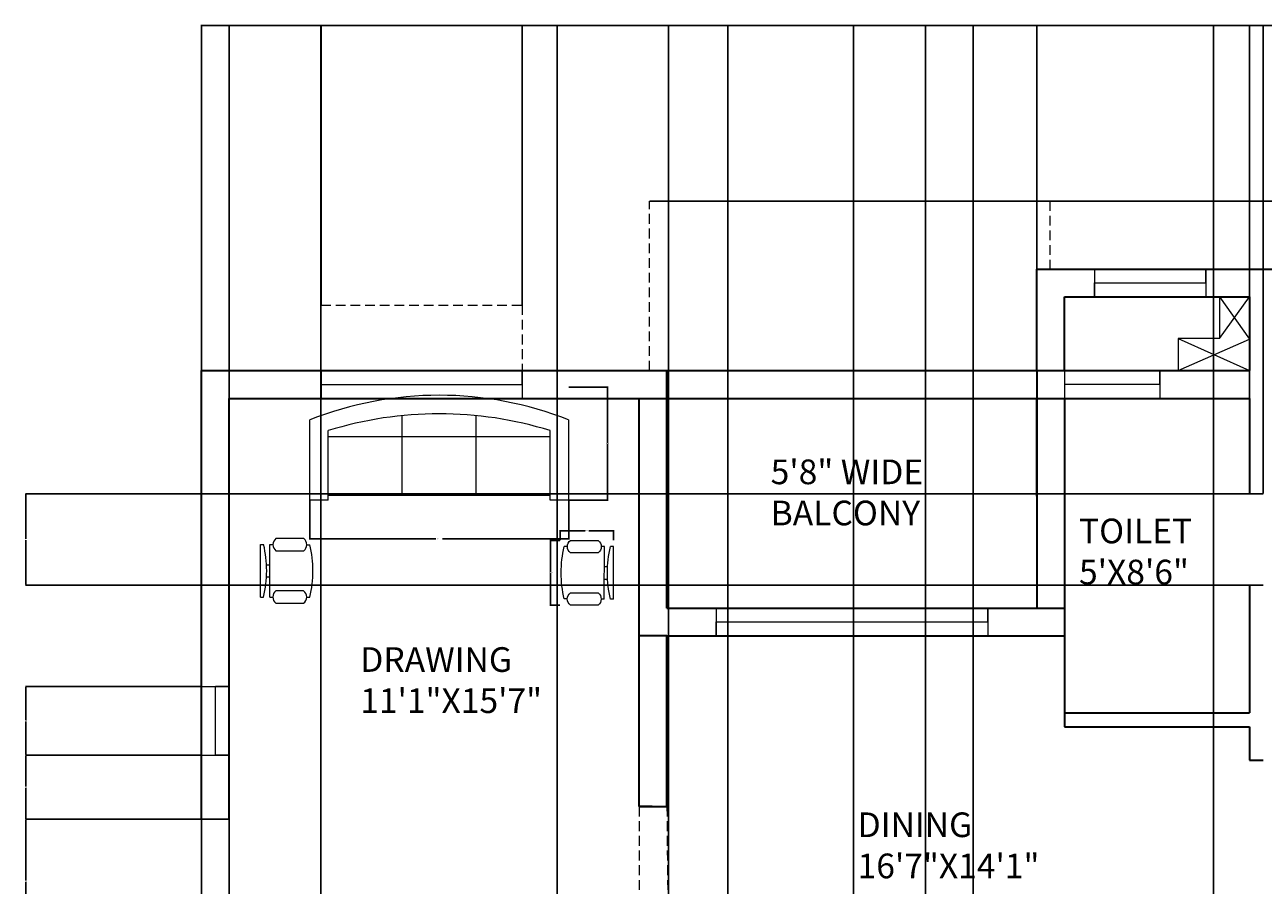
# Model space of a CAD drawing. Units: inches. Extents: x 276 to 912, y -567 to 621.
# Tile 6 of 7: x 276 to 678, y 342 to 621. Entities that reach past the tile are written whole.
import ezdxf

# ---------------------------------------------------------------- set-up
doc = ezdxf.new("R2010")
doc.units = ezdxf.units.IN
doc.linetypes.add('HIDDEN2', pattern=[4.7625, 3.175, -1.5875])
for name, color, linetype, lineweight in [('A-ANNO-DIMS', 2, 'Continuous', 18), ('A-AREA-IDEN', 7, 'Continuous', 18), ('A-DOOR', 3, 'Continuous', 25), ('A-FLOR-OVHD', 8, 'HIDDEN2', 13), ('A-FLOR-SHFT', 8, 'Continuous', 18), ('A-FURN', 8, 'Continuous', 18), ('A-GLAZ', 4, 'Continuous', 18), ('A-WALL', 7, 'Continuous', 35), ('A-WALL-HIDN', 8, 'HIDDEN2', 18)]:
    doc.layers.add(name, color=color, linetype=linetype, lineweight=lineweight)
doc.dimstyles.get("Standard").update_dxf_attribs({"dimtxt": 0.18, "dimasz": 0.18, "dimexe": 0.18, "dimexo": 0.0625, "dimgap": 0.09, "dimtad": 0, "dimtih": 1, "dimtoh": 1, "dimdec": 4, "dimzin": 0, "dimdsep": 46, "dimtxsty": 'Standard', "dimcen": 0.09, "dimadec": 0, "dimazin": 0, "dimtfac": 1, "dimtdec": 4, "dimtofl": 0, "dimtmove": 0, "dimatfit": 3, "dimfxl": 1, "dimtolj": 1, "dimtzin": 0, "dimarcsym": 0})

# ---------------------------------------------------------------- blocks, each defined once
blk = doc.blocks.new('Chair - Desk')
for p, q in [((-8.5, 0), (-8.5, -1)), ((-8.5, 0), (8.5, 0)), ((8.5, 0), (8.5, -1)), ((-8.5, -3), (-8.5, -4)), ((-8.5, -3), (8.5, -3)), ((-2, -3), (-2, -1.9355)), ((2, -1.9576), (2, -3)), ((8.5, -3), (8.5, -4)), ((-10.5, -5), (-10.5, -14)), ((-6.5, -14), (-6.5, -5)), ((6.5, -5), (6.5, -14)), ((10.5, -14), (10.5, -5)), ((-8.5, -15), (-8.5, -16)), ((8.5, -15), (8.5, -16))]:
    blk.add_line(p, q)
for centre, radius, start, end in [((-8.5, -6.5), 2.5, 36.8699, 143.1301), ((0, 34.625), 36.625, 256.5803, 283.4197), ((8.5, -6.5), 2.5, 36.8699, 143.1301), ((-8.5, -12.5), 2.5, 216.8699, 323.1301), ((0, 19.625), 36.625, 256.5803, 283.4197), ((8.5, -12.5), 2.5, 216.8699, 323.1301)]:
    blk.add_arc(centre, radius, start, end)
blk = doc.blocks.new('Sofa - Roundback 7 ft.')
for p, q in [((-12.00002, -32.4421), (-12.00003, -6.5971)), ((11.99997, -32.4421), (11.99998, -6.5971)), ((-36.000027, -34), (-36.000027, -11.4696)), ((35.99998, -34), (35.99998, -11.4696)), ((-35.999844, -13.3819), (35.9998, -13.3819)), ((-36.000027, -32.4421), (35.99998, -32.4421))]:
    blk.add_line(p, q)
for points in [[(-36.000027, -34), (-42.000027, -34), (-42.000027, -8)], [(41.99998, -8), (41.99998, -34), (35.99998, -34)]]:
    blk.add_lwpolyline(points)
for centre, radius, start, end in [((0, -114.25), 114.25, 68.43141, 111.5686), ((-0.00001, -127.1968), 121.1968, 72.72033, 107.2797)]:
    blk.add_arc(centre, radius, start, end)
blk = doc.blocks.new('DOOR-JAMB-4.5IN')
for p, q in [((0, 2.25), (0, 4.5)), ((0, 4.5), (0, 0))]:
    blk.add_line(p, q)
blk = doc.blocks.new('DOOR-JAMB-9IN')
for p, q in [((4.5, 0), (0, 0)), ((0, 0), (9, 0))]:
    blk.add_line(p, q)
blk = doc.blocks.new('*D14')
at = {"layer": 'A-ANNO-DIMS', "color": 0, "lineweight": -2, "transparency": 16777216}
for p, q in [((449.38, 454.26), (446.12, 454.27)), ((446.3, 454.09), (446.28, 443.95)), ((446.27, 433.45), (446.28, 443.59)), ((449.35, 433.26), (446.09, 433.27))]:
    blk.add_line(p, q, dxfattribs=at)
at = {"layer": 'A-ANNO-DIMS', "color": 0, "transparency": 16777216}
for points in [[(446.27, 454.09), (446.33, 454.09), (446.3, 454.27)], [(446.24, 433.45), (446.3, 433.45), (446.27, 433.27)]]:
    blk.add_solid(points, dxfattribs=at)
at = {"layer": 'Defpoints', "color": 0, "transparency": 16777216}
for p in [(446.3, 454.27), (449.45, 454.26), (449.42, 433.26)]:
    blk.add_point(p, dxfattribs=at)
at = {"layer": 'A-ANNO-DIMS', "color": 0, "transparency": 16777216, "insert": (446.28, 443.77), "char_height": 0.18, "attachment_point": 5}
blk.add_mtext('\\A1;CHAIR 21 TYP.', dxfattribs=at)
blk = doc.blocks.new('*D15')
at = {"layer": 'A-ANNO-DIMS', "color": 0, "lineweight": -2, "transparency": 16777216}
for p, q in [((449.45, 454.33), (449.45, 457.59)), ((449.63, 457.41), (457.52, 457.4)), ((466.6, 457.39), (458.72, 457.4)), ((466.78, 454.3), (466.78, 457.57))]:
    blk.add_line(p, q, dxfattribs=at)
at = {"layer": 'A-ANNO-DIMS', "color": 0, "transparency": 16777216}
for points in [[(449.63, 457.44), (449.63, 457.38), (449.45, 457.41)], [(466.6, 457.42), (466.6, 457.36), (466.78, 457.39)]]:
    blk.add_solid(points, dxfattribs=at)
at = {"layer": 'Defpoints', "color": 0, "transparency": 16777216}
for p in [(449.45, 454.26), (466.78, 457.39), (466.78, 454.24)]:
    blk.add_point(p, dxfattribs=at)
at = {"layer": 'A-ANNO-DIMS', "color": 0, "transparency": 16777216, "insert": (458.12, 457.4), "char_height": 0.18, "attachment_point": 5}
blk.add_mtext('\\A1;17 TYP.', dxfattribs=at)
blk = doc.blocks.new('*D20')
at = {"layer": 'A-ANNO-DIMS', "color": 0, "lineweight": -2, "transparency": 16777216}
for p, q in [((368.2, 467.26), (368.2, 454.55)), ((452.2, 467.26), (452.2, 454.55)), ((368.38, 454.73), (409.12, 454.73)), ((452.02, 454.73), (411.28, 454.73))]:
    blk.add_line(p, q, dxfattribs=at)
at = {"layer": 'A-ANNO-DIMS', "color": 0, "transparency": 16777216}
for points in [[(368.38, 454.76), (368.38, 454.7), (368.2, 454.73)], [(452.02, 454.76), (452.02, 454.7), (452.2, 454.73)]]:
    blk.add_solid(points, dxfattribs=at)
at = {"layer": 'Defpoints', "color": 0, "transparency": 16777216}
for p in [(368.2, 467.33), (452.2, 467.33), (452.2, 454.73)]:
    blk.add_point(p, dxfattribs=at)
at = {"layer": 'A-ANNO-DIMS', "color": 0, "transparency": 16777216, "insert": (410.2, 454.73), "char_height": 0.18, "attachment_point": 5}
blk.add_mtext('\\A1;SOFA 84 TYP.', dxfattribs=at)
blk = doc.blocks.new('*D21')
at = {"layer": 'A-ANNO-DIMS', "color": 0, "lineweight": -2, "transparency": 16777216}
for p, q in [((452.26, 503.99), (464.98, 503.99)), ((464.8, 503.81), (464.8, 485.84)), ((464.8, 467.51), (464.8, 485.48)), ((452.26, 467.33), (464.98, 467.33))]:
    blk.add_line(p, q, dxfattribs=at)
at = {"layer": 'A-ANNO-DIMS', "color": 0, "transparency": 16777216}
for points in [[(464.77, 503.81), (464.83, 503.81), (464.8, 503.99)], [(464.77, 467.51), (464.83, 467.51), (464.8, 467.33)]]:
    blk.add_solid(points, dxfattribs=at)
at = {"layer": 'Defpoints', "color": 0, "transparency": 16777216}
for p in [(452.2, 503.99), (464.8, 503.99), (452.2, 467.33)]:
    blk.add_point(p, dxfattribs=at)
at = {"layer": 'A-ANNO-DIMS', "color": 0, "transparency": 16777216, "insert": (464.8, 485.66), "char_height": 0.18, "attachment_point": 5}
blk.add_mtext('\\A1;37 TYP.', dxfattribs=at)
blk = doc.blocks.new('*D25')
at = {"layer": 'A-ANNO-DIMS', "color": 0, "lineweight": -2, "transparency": 16777216}
for p, q in [((478.5, 564.29), (911.39, 564.29)), ((911.21, 564.11), (911.21, 34.31)), ((911.21, -495.86), (911.21, 33.95)), ((582.98, -496.04), (911.39, -496.04))]:
    blk.add_line(p, q, dxfattribs=at)
at = {"layer": 'A-ANNO-DIMS', "color": 0, "transparency": 16777216}
for points in [[(911.18, 564.11), (911.24, 564.11), (911.21, 564.29)], [(911.18, -495.86), (911.24, -495.86), (911.21, -496.04)]]:
    blk.add_solid(points, dxfattribs=at)
at = {"layer": 'Defpoints', "color": 0, "transparency": 16777216}
for p in [(478.44, 564.29), (582.92, -496.04), (911.21, -496.04)]:
    blk.add_point(p, dxfattribs=at)
at = {"layer": 'A-ANNO-DIMS', "color": 0, "transparency": 16777216, "insert": (911.21, 34.13), "char_height": 0.18, "attachment_point": 5}
blk.add_mtext('\\A1;1060.3', dxfattribs=at)
blk = doc.blocks.new('*D27')
at = {"layer": 'A-ANNO-DIMS', "color": 0, "lineweight": -2, "transparency": 16777216}
for p, q in [((333.082179, 509.380751), (333.082179, 621.473746)), ((333.262179, 621.293746), (468.282179, 621.293746)), ((603.902179, 621.293746), (468.882179, 621.293746)), ((604.082179, 542.322551), (604.082179, 621.473746))]:
    blk.add_line(p, q, dxfattribs=at)
at = {"layer": 'A-ANNO-DIMS', "color": 0, "transparency": 16777216}
for points in [[(333.262179, 621.323746), (333.262179, 621.263746), (333.082179, 621.293746)], [(603.902179, 621.323746), (603.902179, 621.263746), (604.082179, 621.293746)]]:
    blk.add_solid(points, dxfattribs=at)
at = {"layer": 'Defpoints', "color": 0, "transparency": 16777216}
for p in [(604.082179, 621.293746), (604.082179, 542.260051), (333.082179, 509.318251)]:
    blk.add_point(p, dxfattribs=at)
at = {"layer": 'A-ANNO-DIMS', "color": 0, "transparency": 16777216, "insert": (468.582179, 621.293746), "char_height": 0.18, "attachment_point": 5}
blk.add_mtext('\\A1;271', dxfattribs=at)
blk = doc.blocks.new('*D28')
at = {"layer": 'A-ANNO-DIMS', "color": 0, "lineweight": -2, "transparency": 16777216}
for p, q in [((604.082179, 542.322551), (604.082179, 621.473746)), ((604.262179, 621.293746), (642.842179, 621.293746)), ((681.902179, 621.293746), (643.322179, 621.293746)), ((682.082179, 542.322551), (682.082179, 621.473746))]:
    blk.add_line(p, q, dxfattribs=at)
at = {"layer": 'A-ANNO-DIMS', "color": 0, "transparency": 16777216}
for points in [[(604.262179, 621.323746), (604.262179, 621.263746), (604.082179, 621.293746)], [(681.902179, 621.323746), (681.902179, 621.263746), (682.082179, 621.293746)]]:
    blk.add_solid(points, dxfattribs=at)
at = {"layer": 'Defpoints', "color": 0, "transparency": 16777216}
for p in [(682.082179, 621.293746), (604.082179, 542.260051), (682.082179, 542.260051)]:
    blk.add_point(p, dxfattribs=at)
at = {"layer": 'A-ANNO-DIMS', "color": 0, "transparency": 16777216, "insert": (643.082179, 621.293746), "char_height": 0.18, "attachment_point": 5}
blk.add_mtext('\\A1;78', dxfattribs=at)
blk = doc.blocks.new('*D37')
at = {"layer": 'A-ANNO-DIMS', "color": 0, "lineweight": -2, "transparency": 16777216}
for p, q in [((333.019679, 363.831643), (275.902179, 363.831643)), ((276.082179, 363.651643), (276.082179, 343.929428)), ((276.082179, 323.847213), (276.082179, 343.569428)), ((333.019679, 323.667213), (275.902179, 323.667213))]:
    blk.add_line(p, q, dxfattribs=at)
at = {"layer": 'A-ANNO-DIMS', "color": 0, "transparency": 16777216}
for points in [[(276.052179, 363.651643), (276.112179, 363.651643), (276.082179, 363.831643)], [(276.052179, 323.847213), (276.112179, 323.847213), (276.082179, 323.667213)]]:
    blk.add_solid(points, dxfattribs=at)
at = {"layer": 'Defpoints', "color": 0, "transparency": 16777216}
for p in [(276.082179, 363.831643), (333.082179, 363.831643), (333.082179, 323.667213)]:
    blk.add_point(p, dxfattribs=at)
at = {"layer": 'A-ANNO-DIMS', "color": 0, "transparency": 16777216, "insert": (276.082179, 343.749428), "char_height": 0.18, "attachment_point": 5}
blk.add_mtext('\\A1;40.164', dxfattribs=at)
blk = doc.blocks.new('*D39')
at = {"layer": 'A-ANNO-DIMS', "color": 0, "lineweight": -2, "transparency": 16777216}
for p, q in [((673.019679, 469.398472), (275.902179, 469.398472)), ((276.082179, 469.218472), (276.082179, 454.742779)), ((276.082179, 439.907086), (276.082179, 454.382779)), ((673.019679, 439.727086), (275.902179, 439.727086))]:
    blk.add_line(p, q, dxfattribs=at)
at = {"layer": 'A-ANNO-DIMS', "color": 0, "transparency": 16777216}
for points in [[(276.052179, 469.218472), (276.112179, 469.218472), (276.082179, 469.398472)], [(276.052179, 439.907086), (276.112179, 439.907086), (276.082179, 439.727086)]]:
    blk.add_solid(points, dxfattribs=at)
at = {"layer": 'Defpoints', "color": 0, "transparency": 16777216}
for p in [(276.082179, 469.398472), (673.082179, 469.398472), (673.082179, 439.727086)]:
    blk.add_point(p, dxfattribs=at)
at = {"layer": 'A-ANNO-DIMS', "color": 0, "transparency": 16777216, "insert": (276.082179, 454.562779), "char_height": 0.18, "attachment_point": 5}
blk.add_mtext('\\A1;29.67', dxfattribs=at)
blk = doc.blocks.new('*D40')
at = {"layer": 'A-ANNO-DIMS', "color": 0, "lineweight": -2, "transparency": 16777216}
for p, q in [((673.082179, 469.460972), (673.082179, 621.473746)), ((673.262179, 621.293746), (675.062179, 621.293746)), ((677.402179, 621.293746), (675.602179, 621.293746)), ((677.582179, 469.460972), (677.582179, 621.473746))]:
    blk.add_line(p, q, dxfattribs=at)
at = {"layer": 'A-ANNO-DIMS', "color": 0, "transparency": 16777216}
for points in [[(673.262179, 621.323746), (673.262179, 621.263746), (673.082179, 621.293746)], [(677.402179, 621.323746), (677.402179, 621.263746), (677.582179, 621.293746)]]:
    blk.add_solid(points, dxfattribs=at)
at = {"layer": 'Defpoints', "color": 0, "transparency": 16777216}
for p in [(677.582179, 621.293746), (673.082179, 469.398472), (677.582179, 469.398472)]:
    blk.add_point(p, dxfattribs=at)
at = {"layer": 'A-ANNO-DIMS', "color": 0, "transparency": 16777216, "insert": (675.332179, 621.293746), "char_height": 0.18, "attachment_point": 5}
blk.add_mtext('\\A1;4.5', dxfattribs=at)
blk = doc.blocks.new('*D41')
at = {"layer": 'A-ANNO-DIMS', "color": 0, "lineweight": -2, "transparency": 16777216}
for p, q in [((333.082179, 363.769143), (333.082179, -553.223061)), ((342.082179, 363.769143), (342.082179, -553.223061)), ((333.262179, -553.043061), (337.432179, -553.043061)), ((341.902179, -553.043061), (337.732179, -553.043061))]:
    blk.add_line(p, q, dxfattribs=at)
at = {"layer": 'A-ANNO-DIMS', "color": 0, "transparency": 16777216}
for points in [[(333.262179, -553.013061), (333.262179, -553.073061), (333.082179, -553.043061)], [(341.902179, -553.013061), (341.902179, -553.073061), (342.082179, -553.043061)]]:
    blk.add_solid(points, dxfattribs=at)
at = {"layer": 'Defpoints', "color": 0, "transparency": 16777216}
for p in [(333.082179, 363.831643), (342.082179, 363.831643), (342.082179, -553.043061)]:
    blk.add_point(p, dxfattribs=at)
at = {"layer": 'A-ANNO-DIMS', "color": 0, "transparency": 16777216, "insert": (337.582179, -553.043061), "char_height": 0.18, "attachment_point": 5}
blk.add_mtext('\\A1;9', dxfattribs=at)
blk = doc.blocks.new('*D42')
at = {"layer": 'A-ANNO-DIMS', "color": 0, "lineweight": -2, "transparency": 16777216}
for p, q in [((484.582179, 267.783946), (484.582179, 621.473746)), ((484.762179, 621.293746), (514.357179, 621.293746)), ((544.402179, 621.293746), (514.807179, 621.293746)), ((544.582179, 267.783946), (544.582179, 621.473746))]:
    blk.add_line(p, q, dxfattribs=at)
at = {"layer": 'A-ANNO-DIMS', "color": 0, "transparency": 16777216}
for points in [[(484.762179, 621.323746), (484.762179, 621.263746), (484.582179, 621.293746)], [(544.402179, 621.323746), (544.402179, 621.263746), (544.582179, 621.293746)]]:
    blk.add_solid(points, dxfattribs=at)
at = {"layer": 'Defpoints', "color": 0, "transparency": 16777216}
for p in [(544.582179, 621.293746), (484.582179, 267.721446), (544.582179, 267.721446)]:
    blk.add_point(p, dxfattribs=at)
at = {"layer": 'A-ANNO-DIMS', "color": 0, "transparency": 16777216, "insert": (514.582179, 621.293746), "char_height": 0.18, "attachment_point": 5}
blk.add_mtext('\\A1;60', dxfattribs=at)
blk = doc.blocks.new('*D44')
at = {"layer": 'A-ANNO-DIMS', "color": 0, "lineweight": -2, "transparency": 16777216}
for p, q in [((333.08, 509.38), (333.08, 621.47)), ((333.26, 621.29), (352.02, 621.29)), ((371.68, 621.29), (352.92, 621.29)), ((371.86, 530.6), (371.86, 621.47))]:
    blk.add_line(p, q, dxfattribs=at)
at = {"layer": 'A-ANNO-DIMS', "color": 0, "transparency": 16777216}
for points in [[(333.26, 621.32), (333.26, 621.26), (333.08, 621.29)], [(371.68, 621.32), (371.68, 621.26), (371.86, 621.29)]]:
    blk.add_solid(points, dxfattribs=at)
at = {"layer": 'Defpoints', "color": 0, "transparency": 16777216}
for p in [(371.86, 621.29), (371.86, 530.54), (333.08, 509.32)]:
    blk.add_point(p, dxfattribs=at)
at = {"layer": 'A-ANNO-DIMS', "color": 0, "transparency": 16777216, "insert": (352.47, 621.29), "char_height": 0.18, "attachment_point": 5}
blk.add_mtext('\\A1;38.78', dxfattribs=at)
blk = doc.blocks.new('*D45')
at = {"layer": 'A-ANNO-DIMS', "color": 0, "lineweight": -2, "transparency": 16777216}
for p, q in [((371.863208, 530.602563), (371.863208, 621.473746)), ((372.043208, 621.293746), (404.102886, 621.293746)), ((436.882564, 621.293746), (404.822886, 621.293746)), ((437.062564, 530.602563), (437.062564, 621.473746))]:
    blk.add_line(p, q, dxfattribs=at)
at = {"layer": 'A-ANNO-DIMS', "color": 0, "transparency": 16777216}
for points in [[(372.043208, 621.323746), (372.043208, 621.263746), (371.863208, 621.293746)], [(436.882564, 621.323746), (436.882564, 621.263746), (437.062564, 621.293746)]]:
    blk.add_solid(points, dxfattribs=at)
at = {"layer": 'Defpoints', "color": 0, "transparency": 16777216}
for p in [(437.062564, 621.293746), (371.863208, 530.540063), (437.062564, 530.540063)]:
    blk.add_point(p, dxfattribs=at)
at = {"layer": 'A-ANNO-DIMS', "color": 0, "transparency": 16777216, "insert": (404.462886, 621.293746), "char_height": 0.18, "attachment_point": 5}
blk.add_mtext('\\A1;65.2', dxfattribs=at)
blk = doc.blocks.new('*D52')
at = {"layer": 'A-ANNO-DIMS', "color": 0, "lineweight": -2, "transparency": 16777216}
for p, q in [((333.019679, 384.618373), (275.902179, 384.618373)), ((276.082179, 384.438373), (276.082179, 374.405008)), ((276.082179, 364.011643), (276.082179, 374.045008)), ((333.019679, 363.831643), (275.902179, 363.831643))]:
    blk.add_line(p, q, dxfattribs=at)
at = {"layer": 'A-ANNO-DIMS', "color": 0, "transparency": 16777216}
for points in [[(276.052179, 384.438373), (276.112179, 384.438373), (276.082179, 384.618373)], [(276.052179, 364.011643), (276.112179, 364.011643), (276.082179, 363.831643)]]:
    blk.add_solid(points, dxfattribs=at)
at = {"layer": 'Defpoints', "color": 0, "transparency": 16777216}
for p in [(276.082179, 384.618373), (333.082179, 384.618373), (333.082179, 363.831643)]:
    blk.add_point(p, dxfattribs=at)
at = {"layer": 'A-ANNO-DIMS', "color": 0, "transparency": 16777216, "insert": (276.082179, 374.225008), "char_height": 0.18, "attachment_point": 5}
blk.add_mtext('\\A1;20.787', dxfattribs=at)
blk = doc.blocks.new('*D53')
at = {"layer": 'A-ANNO-DIMS', "color": 0, "lineweight": -2, "transparency": 16777216}
for p, q in [((333.02, 406.87), (275.9, 406.87)), ((276.08, 406.69), (276.08, 395.92)), ((276.08, 384.8), (276.08, 395.56)), ((333.02, 384.62), (275.9, 384.62))]:
    blk.add_line(p, q, dxfattribs=at)
at = {"layer": 'A-ANNO-DIMS', "color": 0, "transparency": 16777216}
for points in [[(276.05, 406.69), (276.11, 406.69), (276.08, 406.87)], [(276.05, 384.8), (276.11, 384.8), (276.08, 384.62)]]:
    blk.add_solid(points, dxfattribs=at)
at = {"layer": 'Defpoints', "color": 0, "transparency": 16777216}
for p in [(276.08, 406.87), (333.08, 406.87), (333.08, 384.62)]:
    blk.add_point(p, dxfattribs=at)
at = {"layer": 'A-ANNO-DIMS', "color": 0, "transparency": 16777216, "insert": (276.08, 395.74), "char_height": 0.18, "attachment_point": 5}
blk.add_mtext('\\A1;22.253', dxfattribs=at)
blk = doc.blocks.new('*D59')
at = {"layer": 'A-ANNO-DIMS', "color": 0, "lineweight": -2, "transparency": 16777216}
for p, q in [((333.082179, -81.315568), (333.082179, 621.473746)), ((333.262179, 621.293746), (457.725334, 621.293746)), ((583.238489, 621.293746), (458.775334, 621.293746)), ((583.418489, -30.671128), (583.418489, 621.473746))]:
    blk.add_line(p, q, dxfattribs=at)
at = {"layer": 'A-ANNO-DIMS', "color": 0, "transparency": 16777216}
for points in [[(333.262179, 621.323746), (333.262179, 621.263746), (333.082179, 621.293746)], [(583.238489, 621.323746), (583.238489, 621.263746), (583.418489, 621.293746)]]:
    blk.add_solid(points, dxfattribs=at)
at = {"layer": 'Defpoints', "color": 0, "transparency": 16777216}
for p in [(583.418489, 621.293746), (583.418489, -30.733628), (333.082179, -81.378068)]:
    blk.add_point(p, dxfattribs=at)
at = {"layer": 'A-ANNO-DIMS', "color": 0, "transparency": 16777216, "insert": (458.250334, 621.293746), "char_height": 0.18, "attachment_point": 5}
blk.add_mtext('\\A1;250.34', dxfattribs=at)
blk = doc.blocks.new('*D60')
at = {"layer": 'A-ANNO-DIMS', "color": 0, "lineweight": -2, "transparency": 16777216}
for p, q in [((583.418489, -30.671128), (583.418489, 621.473746)), ((583.598489, 621.293746), (622.178489, 621.293746)), ((661.238489, 621.293746), (622.658489, 621.293746)), ((661.418489, -30.671128), (661.418489, 621.473746))]:
    blk.add_line(p, q, dxfattribs=at)
at = {"layer": 'A-ANNO-DIMS', "color": 0, "transparency": 16777216}
for points in [[(583.598489, 621.323746), (583.598489, 621.263746), (583.418489, 621.293746)], [(661.238489, 621.323746), (661.238489, 621.263746), (661.418489, 621.293746)]]:
    blk.add_solid(points, dxfattribs=at)
at = {"layer": 'Defpoints', "color": 0, "transparency": 16777216}
for p in [(661.418489, 621.293746), (583.418489, -30.733628), (661.418489, -30.733628)]:
    blk.add_point(p, dxfattribs=at)
at = {"layer": 'A-ANNO-DIMS', "color": 0, "transparency": 16777216, "insert": (622.418489, 621.293746), "char_height": 0.18, "attachment_point": 5}
blk.add_mtext('\\A1;78', dxfattribs=at)
blk = doc.blocks.new('*D61')
at = {"layer": 'A-ANNO-DIMS', "color": 0, "lineweight": -2, "transparency": 16777216}
for p, q in [((661.418489, -30.671128), (661.418489, 621.473746)), ((661.598489, 621.293746), (741.263489, 621.293746)), ((821.738489, 621.293746), (742.073489, 621.293746)), ((821.918489, -64.479004), (821.918489, 621.473746))]:
    blk.add_line(p, q, dxfattribs=at)
at = {"layer": 'A-ANNO-DIMS', "color": 0, "transparency": 16777216}
for points in [[(661.598489, 621.323746), (661.598489, 621.263746), (661.418489, 621.293746)], [(821.738489, 621.323746), (821.738489, 621.263746), (821.918489, 621.293746)]]:
    blk.add_solid(points, dxfattribs=at)
at = {"layer": 'Defpoints', "color": 0, "transparency": 16777216}
for p in [(821.918489, 621.293746), (661.418489, -30.733628), (821.918489, -64.541504)]:
    blk.add_point(p, dxfattribs=at)
at = {"layer": 'A-ANNO-DIMS', "color": 0, "transparency": 16777216, "insert": (741.668489, 621.293746), "char_height": 0.18, "attachment_point": 5}
blk.add_mtext('\\A1;160.5', dxfattribs=at)
blk = doc.blocks.new('*D65')
at = {"layer": 'A-ANNO-DIMS', "color": 0, "lineweight": -2, "transparency": 16777216}
for p, q in [((342.08, -229.93), (342.08, 621.47)), ((342.26, 621.29), (356.48, 621.29)), ((371.59, 621.29), (357.38, 621.29)), ((371.77, -229.93), (371.77, 621.47))]:
    blk.add_line(p, q, dxfattribs=at)
at = {"layer": 'A-ANNO-DIMS', "color": 0, "transparency": 16777216}
for points in [[(342.26, 621.32), (342.26, 621.26), (342.08, 621.29)], [(371.59, 621.32), (371.59, 621.26), (371.77, 621.29)]]:
    blk.add_solid(points, dxfattribs=at)
at = {"layer": 'Defpoints', "color": 0, "transparency": 16777216}
for p in [(371.77, 621.29), (342.08, -229.99), (371.77, -229.99)]:
    blk.add_point(p, dxfattribs=at)
at = {"layer": 'A-ANNO-DIMS', "color": 0, "transparency": 16777216, "insert": (356.93, 621.29), "char_height": 0.18, "attachment_point": 5}
blk.add_mtext('\\A1;29.69', dxfattribs=at)
blk = doc.blocks.new('*D70')
at = {"layer": 'A-ANNO-DIMS', "color": 0, "lineweight": -2, "transparency": 16777216}
for p, q in [((448.42, -73.48), (448.42, 621.47)), ((448.6, 621.29), (475.69, 621.29)), ((503.69, 621.29), (476.59, 621.29)), ((503.87, -45.06), (503.87, 621.47))]:
    blk.add_line(p, q, dxfattribs=at)
at = {"layer": 'A-ANNO-DIMS', "color": 0, "transparency": 16777216}
for points in [[(448.6, 621.32), (448.6, 621.26), (448.42, 621.29)], [(503.69, 621.32), (503.69, 621.26), (503.87, 621.29)]]:
    blk.add_solid(points, dxfattribs=at)
at = {"layer": 'Defpoints', "color": 0, "transparency": 16777216}
for p in [(503.87, 621.29), (503.87, -45.12), (448.42, -73.54)]:
    blk.add_point(p, dxfattribs=at)
at = {"layer": 'A-ANNO-DIMS', "color": 0, "transparency": 16777216, "insert": (476.14, 621.29), "char_height": 0.18, "attachment_point": 5}
blk.add_mtext('\\A1;55.45', dxfattribs=at)
blk = doc.blocks.new('*D71')
at = {"layer": 'A-ANNO-DIMS', "color": 0, "lineweight": -2, "transparency": 16777216}
for p, q in [((503.866476, -45.059003), (503.866476, 621.473746)), ((504.046476, 621.293746), (535.522963, 621.293746)), ((567.83945, 621.293746), (536.362963, 621.293746)), ((568.01945, -45.059003), (568.01945, 621.473746))]:
    blk.add_line(p, q, dxfattribs=at)
at = {"layer": 'A-ANNO-DIMS', "color": 0, "transparency": 16777216}
for points in [[(504.046476, 621.323746), (504.046476, 621.263746), (503.866476, 621.293746)], [(567.83945, 621.323746), (567.83945, 621.263746), (568.01945, 621.293746)]]:
    blk.add_solid(points, dxfattribs=at)
at = {"layer": 'Defpoints', "color": 0, "transparency": 16777216}
for p in [(568.01945, 621.293746), (503.866476, -45.121503), (568.01945, -45.121503)]:
    blk.add_point(p, dxfattribs=at)
at = {"layer": 'A-ANNO-DIMS', "color": 0, "transparency": 16777216, "insert": (535.942963, 621.293746), "char_height": 0.18, "attachment_point": 5}
blk.add_mtext('\\A1;64.15', dxfattribs=at)

msp = doc.modelspace()

# ---------------------------------------------------------------- linework, layer by layer
at = {"layer": 'A-FLOR-OVHD'}
for p, q in [((478.4357, 509.3183), (478.4357, 564.2937)), ((478.4357, 564.2937), (608.356, 564.2937)), ((608.356, 564.2937), (608.356, 542.2601)), ((371.8632, 509.3183), (371.8632, 530.5401)), ((371.8632, 530.5401), (437.0626, 530.5401)), ((437.0626, 530.5401), (437.0626, 507.0683))]:
    msp.add_line(p, q, dxfattribs=at)
at = {"layer": 'A-FLOR-SHFT'}
for p, q in [((663.4395, 533.2601), (663.4395, 519.7905)), ((663.4395, 533.2601), (673.0822, 519.5713)), ((663.4395, 519.7905), (673.0822, 533.2601)), ((663.4395, 519.7905), (649.9445, 519.7905)), ((649.9445, 519.7905), (649.9445, 509.3183)), ((649.9445, 519.7905), (673.0822, 509.3183)), ((649.9445, 509.3183), (673.0822, 519.5713))]:
    msp.add_line(p, q, dxfattribs=at)
at = {"layer": 'A-GLAZ'}
for p, q in [((622.7923, 542.2601), (622.7923, 533.2601)), ((658.9977, 537.7601), (658.9977, 542.2601)), ((658.9977, 542.2601), (658.9977, 533.2601)), ((622.7923, 533.2601), (622.7923, 537.7601)), ((622.7923, 537.7601), (658.9977, 537.7601)), ((371.8632, 509.3183), (371.8632, 500.3183)), ((437.0626, 504.8183), (437.0626, 509.3183)), ((437.0626, 509.3183), (437.0626, 500.3183)), ((613.0822, 509.3183), (613.0822, 496.317)), ((644.0681, 504.9639), (644.0681, 509.3183)), ((644.0681, 509.3183), (644.0681, 500.3183)), ((371.8632, 500.3183), (371.8632, 504.8183)), ((371.8632, 504.8183), (437.0626, 504.8183)), ((613.0822, 504.9639), (644.0681, 504.9639)), ((500.0298, 432.3183), (500.0298, 423.3183)), ((588.2676, 427.8183), (588.2676, 432.3183)), ((588.2676, 432.3183), (588.2676, 423.3183)), ((500.0298, 423.3183), (500.0298, 427.8183)), ((500.0298, 427.8183), (580.57, 427.8183)), ((580.57, 427.8183), (588.2676, 427.8183)), ((333.0822, 406.8714), (342.0822, 406.8714)), ((342.0822, 406.8714), (337.5822, 406.8714)), ((337.5822, 384.6184), (337.5822, 406.8714)), ((333.0822, 384.6184), (342.0822, 384.6184)), ((342.0822, 384.6184), (337.5822, 384.6184))]:
    msp.add_line(p, q, dxfattribs=at)
at = {"layer": 'A-WALL'}
for p, q in [((604.0822, 542.2601), (682.0822, 542.2601)), ((604.0822, 509.3183), (604.0822, 542.2601)), ((613.0822, 509.3183), (613.0822, 533.2601)), ((613.0822, 533.2601), (673.0822, 533.2601)), ((673.0822, 533.2601), (673.0822, 509.3183)), ((333.0822, 509.3183), (673.0822, 509.3183)), ((333.0822, 363.8316), (333.0822, 509.3183)), ((484.0822, 500.3183), (484.0822, 509.3183)), ((604.0822, 509.3183), (604.0822, 500.3183)), ((342.0822, 500.3183), (673.0822, 500.3183)), ((342.0822, 363.8316), (342.0822, 500.3183)), ((475.0822, 367.9375), (475.0822, 500.3183)), ((484.0822, 432.3183), (484.0822, 500.3183)), ((604.0822, 468.6398), (604.0822, 500.3183)), ((604.0822, 500.3183), (604.0822, 432.3183)), ((613.0822, 500.3183), (613.0822, 432.3183)), ((673.0822, 500.3183), (673.0822, 469.3985)), ((673.0822, 439.7271), (673.0822, 432.3183)), ((484.0822, 432.3183), (613.0822, 432.3183)), ((613.0822, 432.3183), (613.0822, 423.3183)), ((673.0822, 432.3183), (673.0822, 398.3183)), ((484.0822, 423.3183), (475.0822, 423.3183)), ((484.0822, 367.9375), (484.0822, 423.3183)), ((484.0822, 423.3183), (613.0822, 423.3183)), ((613.0822, 423.3183), (613.0822, 393.8183)), ((613.0822, 398.3183), (673.0822, 398.3183)), ((613.0822, 393.8183), (673.0822, 393.8183)), ((673.0822, 393.8183), (673.0822, 382.9782)), ((673.0822, 382.9782), (677.5822, 382.9782)), ((479.3405, 367.9375), (475.0822, 367.9375)), ((475.0822, 367.9375), (484.0822, 367.9375))]:
    msp.add_line(p, q, dxfattribs=at)
at = {"layer": 'A-WALL-HIDN'}
for p, q in [((475.0822, 367.9375), (475.0822, 313.3183)), ((484.0822, 367.9375), (484.5822, 313.3183))]:
    msp.add_line(p, q, dxfattribs=at)

# ---------------------------------------------------------------- block references
at = {"layer": 'A-DOOR'}
for p, rotation in [((673.0819, 469.3985), 270), ((677.5824, 439.727), 90)]:
    msp.add_blockref('DOOR-JAMB-4.5IN', p, dxfattribs=dict(at, rotation=rotation))
msp.add_blockref('DOOR-JAMB-9IN', (333.082, 363.832), dxfattribs=at)
at = {"layer": 'A-FURN'}
msp.add_blockref('Sofa - Roundback 7 ft.', (410.1971, 501.3258), dxfattribs=at)
at = {"layer": 'A-FURN', "rotation": 89.91489374852046}
msp.add_blockref('Chair - Desk', (352.2097, 444.3931), dxfattribs=at)
at = {"layer": 'A-FURN', "xscale": -1, "rotation": 269.9148937485156}
msp.add_blockref('Chair - Desk', (466.7639, 443.7387), dxfattribs=at)

# ---------------------------------------------------------------- texts
at = {"layer": 'A-AREA-IDEN', "char_height": 8, "attachment_point": 1}
for s, insert in [('{\\fTimes New Roman|b0|i0|c0|p18;5\'8" WIDE BALCONY}', (517.7441, 480.4908)), ('{\\fTimes New Roman|b0|i0|c0|p18;TOILET\\P5\'X8\'6"}', (617.8035, 461.3272)), ('{\\fTimes New Roman|b0|i0|c0|p18;DRAWING\\P11\'1"X15\'7"}', (384.5591, 419.6227)), ('{\\fTimes New Roman|b0|i0|c0|p18;DINING\\P16\'7"X14\'1"}', (545.9572, 366.0383))]:
    msp.add_mtext_dynamic_manual_height_columns(s, width=62.274017, gutter_width=12.5, heights=[0], dxfattribs=dict(at, insert=insert))

# ---------------------------------------------------------------- dimensions: what is measured, and where the dimension line sits
at = {"layer": 'A-ANNO-DIMS'}
for base, p1, p2, override, picture, middle in [((604.0822, 621.2937), (333.0822, 509.3183), (604.0822, 542.2601), {"dimdec": 0, "dimlfac": 1, "dimrnd": 0, "dimzin": 0, "dimdsep": 46, "dimlunit": 2}, '*D27', (468.5822, 621.2937)), ((371.8632, 621.2937), (333.0822, 509.3183), (371.8632, 530.5401), {"dimdec": 2, "dimlfac": 1, "dimrnd": 0, "dimzin": 0, "dimdsep": 46, "dimlunit": 2}, '*D44', (352.4727, 621.2937)), ((583.4185, 621.2937), (333.0822, -81.3781), (583.4185, -30.7336), {"dimdec": 2, "dimlfac": 1, "dimrnd": 0, "dimzin": 0, "dimdsep": 46, "dimlunit": 2}, '*D59', (458.2503, 621.2937)), ((371.7724, 621.2937), (342.0822, -229.9899), (371.7724, -229.9899), {"dimdec": 2, "dimlfac": 1, "dimrnd": 0, "dimzin": 0, "dimdsep": 46, "dimlunit": 2}, '*D65', (356.9273, 621.2937)), ((437.0626, 621.2937), (371.8632, 530.5401), (437.0626, 530.5401), {"dimdec": 1, "dimlfac": 1, "dimrnd": 0, "dimzin": 0, "dimdsep": 46, "dimlunit": 2}, '*D45', (404.4629, 621.2937)), ((503.8665, 621.2937), (448.4185, -73.5415), (503.8665, -45.1215), {"dimdec": 2, "dimlfac": 1, "dimrnd": 0, "dimzin": 0, "dimdsep": 46, "dimlunit": 2}, '*D70', (476.1425, 621.2937)), ((544.5822, 621.2937), (484.5822, 267.7214), (544.5822, 267.7214), {"dimdec": 0, "dimlfac": 1, "dimrnd": 0, "dimzin": 0, "dimdsep": 46, "dimlunit": 2}, '*D42', (514.5822, 621.2937)), ((568.0194, 621.2937), (503.8665, -45.1215), (568.0194, -45.1215), {"dimdec": 2, "dimlfac": 1, "dimrnd": 0, "dimzin": 0, "dimdsep": 46, "dimlunit": 2}, '*D71', (535.943, 621.2937)), ((661.4185, 621.2937), (583.4185, -30.7336), (661.4185, -30.7336), {"dimdec": 0, "dimlfac": 1, "dimrnd": 0, "dimzin": 0, "dimdsep": 46, "dimlunit": 2}, '*D60', (622.4185, 621.2937)), ((682.0822, 621.2937), (604.0822, 542.2601), (682.0822, 542.2601), {"dimdec": 0, "dimlfac": 1, "dimrnd": 0, "dimzin": 0, "dimdsep": 46, "dimlunit": 2}, '*D28', (643.0822, 621.2937)), ((821.9185, 621.2937), (661.4185, -30.7336), (821.9185, -64.5415), {"dimdec": 1, "dimlfac": 1, "dimrnd": 0, "dimzin": 0, "dimdsep": 46, "dimlunit": 2}, '*D61', (741.6685, 621.2937)), ((677.5822, 621.2937), (673.0822, 469.3985), (677.5822, 469.3985), {"dimdec": 1, "dimlfac": 1, "dimrnd": 0, "dimzin": 0, "dimdsep": 46, "dimlunit": 2}, '*D40', (675.3322, 621.2937)), ((342.0822, -553.0431), (333.0822, 363.8316), (342.0822, 363.8316), {"dimdec": 0, "dimlfac": 1, "dimrnd": 0, "dimzin": 0, "dimdsep": 46, "dimlunit": 2}, '*D41', (337.5822, -553.0431))]:
    dim = msp.add_linear_dim(base=base, p1=p1, p2=p2, dimstyle='Standard', override=override, dxfattribs=at)
    dim.commit()
    dim.dimension.update_dxf_attribs({"geometry": picture, "text_midpoint": middle})
for base, p1, p2, override, picture, middle in [((911.2091, -496.0431), (478.4357, 564.2937), (582.9185, -496.0431), {"dimdec": 1, "dimlfac": 1, "dimrnd": 0, "dimzin": 0, "dimdsep": 46, "dimlunit": 2}, '*D25', (911.2091, 34.1253)), ((276.0822, 469.3985), (673.0822, 439.7271), (673.0822, 469.3985), {"dimdec": 2, "dimlfac": 1, "dimrnd": 0, "dimzin": 0, "dimdsep": 46, "dimlunit": 2}, '*D39', (276.0822, 454.5628)), ((276.0822, 406.8714), (333.0822, 384.6184), (333.0822, 406.8714), {"dimdec": 3, "dimlfac": 1, "dimrnd": 0, "dimzin": 0, "dimdsep": 46, "dimlunit": 2}, '*D53', (276.0822, 395.7449)), ((276.0822, 384.6184), (333.0822, 363.8316), (333.0822, 384.6184), {"dimdec": 3, "dimlfac": 1, "dimrnd": 0, "dimzin": 0, "dimdsep": 46, "dimlunit": 2}, '*D52', (276.0822, 374.225)), ((276.0822, 363.8316), (333.0822, 323.6672), (333.0822, 363.8316), {"dimdec": 3, "dimlfac": 1, "dimrnd": 0, "dimzin": 0, "dimdsep": 46, "dimlunit": 2}, '*D37', (276.0822, 343.7494))]:
    dim = msp.add_linear_dim(base=base, p1=p1, p2=p2, angle=90, dimstyle='Standard', override=override, dxfattribs=at)
    dim.commit()
    dim.dimension.update_dxf_attribs({"geometry": picture, "text_midpoint": middle})
for base, p1, p2, angle, text, picture, middle in [((464.7971, 503.9925), (452.1971, 467.3258), (452.1971, 503.9925), 90, '<> TYP.', '*D21', (464.7971, 485.6592)), ((446.2962, 454.2691), (449.415, 433.2645), (449.4462, 454.2644), 89.914894, 'CHAIR <> TYP.', '*D14', (446.2806, 443.7691)), ((466.7842, 457.3887), (449.4462, 454.2644), (466.7795, 454.2387), 359.914894, '<> TYP.', '*D15', (458.1175, 457.4016))]:
    dim = msp.add_linear_dim(base=base, p1=p1, p2=p2, angle=angle, text=text, dimstyle='Standard', override={"dimdec": 0, "dimlfac": 1, "dimrnd": 0, "dimzin": 0, "dimdsep": 46, "dimlunit": 2}, dxfattribs=at)
    dim.commit()
    dim.dimension.update_dxf_attribs({"geometry": picture, "text_midpoint": middle})
dim = msp.add_linear_dim(base=(452.1971, 454.7258), p1=(368.1971, 467.3258), p2=(452.1971, 467.3258), text='SOFA <> TYP.', dimstyle='Standard', override={"dimdec": 0, "dimlfac": 1, "dimrnd": 0, "dimzin": 0, "dimdsep": 46, "dimlunit": 2}, dxfattribs=at)
dim.commit()
dim.dimension.update_dxf_attribs({"geometry": '*D20', "text_midpoint": (410.1971, 454.7258)})

doc.saveas('drawing.dxf')
